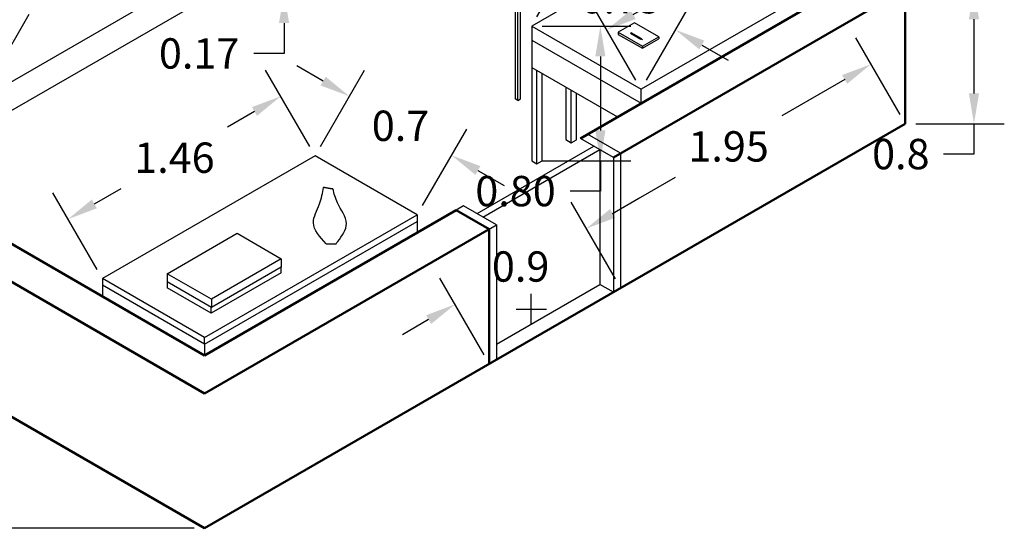
# Model space of a CAD drawing. Units: metres. Extents: x 4633 to 4644.7, y 5356.8 to 5365.2.
# Tile 2 of 3: x 4638.8 to 4644.7, y 5356.8 to 5359.9. Entities that reach past the tile are written whole.
import ezdxf

# ---------------------------------------------------------------- set-up
doc = ezdxf.new("R2010")
doc.units = ezdxf.units.M
for name, color, linetype, lineweight in [('A-ANNO-DIMS', 2, 'Continuous', 18), ('A-DOOR', 4, 'Continuous', 25), ('A-FURN', 8, 'Continuous', 25), ('A-WALL', 7, 'Continuous', 50)]:
    doc.layers.add(name, color=color, linetype=linetype, lineweight=lineweight)
doc.styles.get("Standard").update_dxf_attribs({"font": 'arial.ttf'})
doc.dimstyles.get("Standard").update_dxf_attribs({"dimtxt": 0.18, "dimasz": 0.18, "dimexe": 0.18, "dimexo": 0.0625, "dimgap": 0.09, "dimtad": 0, "dimtih": 1, "dimtoh": 1, "dimdec": 4, "dimzin": 0, "dimdsep": 46, "dimtxsty": 'Standard', "dimcen": 0.09, "dimadec": 0, "dimazin": 0, "dimtfac": 1, "dimtdec": 4, "dimtofl": 0, "dimtmove": 0, "dimatfit": 3, "dimfxl": 1, "dimtolj": 1, "dimtzin": 0, "dimarcsym": 0})

# ---------------------------------------------------------------- blocks, each defined once
blk = doc.blocks.new('*D3')
at = {"layer": 'A-ANNO-DIMS', "color": 0, "lineweight": -2, "transparency": 16777216}
for p, q in [((4639.855, 5364.6413), (4635.6927, 5364.6413)), ((4635.8727, 5364.4613), (4635.8727, 5360.9232)), ((4635.8727, 5357.0213), (4635.8727, 5360.5594)), ((4639.855, 5356.8413), (4635.6927, 5356.8413))]:
    blk.add_line(p, q, dxfattribs=at)
at = {"layer": 'A-ANNO-DIMS', "color": 0, "transparency": 16777216}
for points in [[(4635.8427, 5364.4613), (4635.9027, 5364.4613), (4635.8727, 5364.6413)], [(4635.8427, 5357.0213), (4635.9027, 5357.0213), (4635.8727, 5356.8413)]]:
    blk.add_solid(points, dxfattribs=at)
at = {"layer": 'Defpoints', "color": 0, "transparency": 16777216}
for p in [(4639.9175, 5364.6413), (4635.8727, 5356.8413), (4639.9175, 5356.8413)]:
    blk.add_point(p, dxfattribs=at)
at = {"layer": 'A-ANNO-DIMS', "color": 0, "transparency": 16777216, "insert": (4635.8727, 5360.7413), "char_height": 0.18, "attachment_point": 5}
blk.add_mtext('\\A1;7.8', dxfattribs=at)
blk = doc.blocks.new('*D6')
at = {"layer": 'A-ANNO-DIMS', "color": 0, "lineweight": -2, "transparency": 16777216}
for p, q in [((4644.1369, 5360.0413), (4644.6619, 5360.0413)), ((4644.4819, 5359.8613), (4644.4819, 5359.4213)), ((4644.1369, 5359.2413), (4644.6619, 5359.2413)), ((4644.4819, 5359.2413), (4644.4819, 5359.0613)), ((4644.4819, 5359.0613), (4644.3019, 5359.0613))]:
    blk.add_line(p, q, dxfattribs=at)
at = {"layer": 'A-ANNO-DIMS', "color": 0, "transparency": 16777216}
for points in [[(4644.4519, 5359.8613), (4644.5119, 5359.8613), (4644.4819, 5360.0413)], [(4644.4519, 5359.4213), (4644.5119, 5359.4213), (4644.4819, 5359.2413)]]:
    blk.add_solid(points, dxfattribs=at)
at = {"layer": 'Defpoints', "color": 0, "transparency": 16777216}
for p in [(4644.0744, 5360.0413), (4644.0744, 5359.2413), (4644.4819, 5359.2413)]:
    blk.add_point(p, dxfattribs=at)
at = {"layer": 'A-ANNO-DIMS', "color": 0, "transparency": 16777216, "insert": (4644.0479, 5359.0613), "char_height": 0.18, "attachment_point": 5}
blk.add_mtext('\\A1;0.8', dxfattribs=at)
blk = doc.blocks.new('*D7')
at = {"layer": 'A-ANNO-DIMS', "color": 0, "lineweight": -2, "transparency": 16777216}
for p, q in [((4642.3544, 5358.3204), (4642.0919, 5358.7751)), ((4642.3378, 5358.7092), (4642.4937, 5358.7992)), ((4641.575, 5357.8704), (4641.3125, 5358.3251)), ((4641.2466, 5358.0792), (4641.0907, 5357.9892))]:
    blk.add_line(p, q, dxfattribs=at)
at = {"layer": 'A-ANNO-DIMS', "color": 0, "transparency": 16777216}
for points in [[(4642.3228, 5358.7352), (4642.3528, 5358.6832), (4642.1819, 5358.6192)], [(4641.2316, 5358.1052), (4641.2616, 5358.0532), (4641.4025, 5358.1692)]]:
    blk.add_solid(points, dxfattribs=at)
at = {"layer": 'Defpoints', "color": 0, "transparency": 16777216}
for p in [(4642.1819, 5358.6192), (4642.3857, 5358.2663), (4641.6062, 5357.8163)]:
    blk.add_point(p, dxfattribs=at)
at = {"layer": 'A-ANNO-DIMS', "color": 0, "transparency": 16777216, "insert": (4641.7922, 5358.3942), "char_height": 0.18, "attachment_point": 5}
blk.add_mtext('\\A1;0.9', dxfattribs=at)
blk = doc.blocks.new('*D8')
at = {"layer": 'A-ANNO-DIMS', "color": 0, "lineweight": -2, "transparency": 16777216}
for p, q in [((4644.0432, 5359.2954), (4643.7807, 5359.7501)), ((4643.7148, 5359.5042), (4643.3413, 5359.2886)), ((4642.3378, 5358.7092), (4642.7112, 5358.9248)), ((4642.3544, 5358.3204), (4642.0919, 5358.7751))]:
    blk.add_line(p, q, dxfattribs=at)
at = {"layer": 'A-ANNO-DIMS', "color": 0, "transparency": 16777216}
for points in [[(4643.6998, 5359.5302), (4643.7298, 5359.4782), (4643.8707, 5359.5942)], [(4642.3228, 5358.7352), (4642.3528, 5358.6832), (4642.1819, 5358.6192)]]:
    blk.add_solid(points, dxfattribs=at)
at = {"layer": 'Defpoints', "color": 0, "transparency": 16777216}
for p in [(4643.8707, 5359.5942), (4644.0744, 5359.2413), (4642.3857, 5358.2663)]:
    blk.add_point(p, dxfattribs=at)
at = {"layer": 'A-ANNO-DIMS', "color": 0, "transparency": 16777216, "insert": (4643.0263, 5359.1067), "char_height": 0.18, "attachment_point": 5}
blk.add_mtext('\\A1;1.95', dxfattribs=at)
blk = doc.blocks.new('*D17')
at = {"layer": 'A-ANNO-DIMS', "color": 0, "lineweight": -2, "transparency": 16777216}
for p, q in [((4637.213, 5360.2454), (4637.4755, 5360.7001)), ((4637.5414, 5360.4542), (4637.771, 5360.3216)), ((4638.6308, 5359.8252), (4638.4012, 5359.9578)), ((4638.6142, 5359.4364), (4638.8767, 5359.8911))]:
    blk.add_line(p, q, dxfattribs=at)
at = {"layer": 'A-ANNO-DIMS', "color": 0, "transparency": 16777216}
for points in [[(4637.5564, 5360.4802), (4637.5264, 5360.4282), (4637.3855, 5360.5442)], [(4638.6458, 5359.8512), (4638.6158, 5359.7992), (4638.7867, 5359.7352)]]:
    blk.add_solid(points, dxfattribs=at)
at = {"layer": 'Defpoints', "color": 0, "transparency": 16777216}
for p in [(4637.1817, 5360.1913), (4638.7867, 5359.7352), (4638.583, 5359.3823)]:
    blk.add_point(p, dxfattribs=at)
at = {"layer": 'A-ANNO-DIMS', "color": 0, "transparency": 16777216, "insert": (4638.0861, 5360.1397), "char_height": 0.18, "attachment_point": 5}
blk.add_mtext('\\A1;1.618', dxfattribs=at)
blk = doc.blocks.new('*D18')
at = {"layer": 'A-ANNO-DIMS', "color": 0, "lineweight": -2, "transparency": 16777216}
for p, q in [((4639.9499, 5360.2437), (4639.6874, 5360.6983)), ((4639.6215, 5360.4524), (4639.3762, 5360.3108)), ((4638.5351, 5359.8252), (4638.7804, 5359.9668)), ((4638.5517, 5359.4364), (4638.2892, 5359.8911))]:
    blk.add_line(p, q, dxfattribs=at)
at = {"layer": 'A-ANNO-DIMS', "color": 0, "transparency": 16777216}
for points in [[(4639.6065, 5360.4784), (4639.6365, 5360.4265), (4639.7774, 5360.5424)], [(4638.5201, 5359.8512), (4638.5501, 5359.7992), (4638.3792, 5359.7352)]]:
    blk.add_solid(points, dxfattribs=at)
at = {"layer": 'Defpoints', "color": 0, "transparency": 16777216}
for p in [(4639.7774, 5360.5424), (4639.9812, 5360.1895), (4638.583, 5359.3823)]:
    blk.add_point(p, dxfattribs=at)
at = {"layer": 'A-ANNO-DIMS', "color": 0, "transparency": 16777216, "insert": (4639.0783, 5360.1388), "char_height": 0.18, "attachment_point": 5}
blk.add_mtext('\\A1;1.61', dxfattribs=at)
blk = doc.blocks.new('*D19')
at = {"layer": 'A-ANNO-DIMS', "color": 0, "lineweight": -2, "transparency": 16777216}
for p, q in [((4640.3887, 5360.3695), (4640.3887, 5360.5495)), ((4640.0437, 5360.1895), (4640.5687, 5360.1895)), ((4640.0437, 5360.0182), (4640.5687, 5360.0182)), ((4640.3887, 5359.8382), (4640.3887, 5359.6582)), ((4640.3887, 5359.6582), (4640.2087, 5359.6582))]:
    blk.add_line(p, q, dxfattribs=at)
at = {"layer": 'A-ANNO-DIMS', "color": 0, "transparency": 16777216}
for points in [[(4640.3587, 5360.3695), (4640.4187, 5360.3695), (4640.3887, 5360.1895)], [(4640.3587, 5359.8382), (4640.4187, 5359.8382), (4640.3887, 5360.0182)]]:
    blk.add_solid(points, dxfattribs=at)
at = {"layer": 'Defpoints', "color": 0, "transparency": 16777216}
for p in [(4639.9812, 5360.1895), (4639.9812, 5360.0182), (4640.3887, 5360.0182)]:
    blk.add_point(p, dxfattribs=at)
at = {"layer": 'A-ANNO-DIMS', "color": 0, "transparency": 16777216, "insert": (4639.8849, 5359.6582), "char_height": 0.18, "attachment_point": 5}
blk.add_mtext('\\A1;0.17', dxfattribs=at)
blk = doc.blocks.new('*D25')
at = {"layer": 'A-ANNO-DIMS', "color": 0, "lineweight": -2, "transparency": 16777216}
for p, q in [((4641.9058, 5360.2632), (4641.7499, 5360.3532)), ((4641.8892, 5359.8745), (4642.1517, 5360.3291)), ((4642.5387, 5359.4995), (4642.8012, 5359.9541)), ((4642.8671, 5359.7082), (4643.023, 5359.6182))]:
    blk.add_line(p, q, dxfattribs=at)
at = {"layer": 'A-ANNO-DIMS', "color": 0, "transparency": 16777216}
for points in [[(4641.9208, 5360.2892), (4641.8908, 5360.2373), (4642.0617, 5360.1732)], [(4642.8821, 5359.7342), (4642.8521, 5359.6823), (4642.7112, 5359.7982)]]:
    blk.add_solid(points, dxfattribs=at)
at = {"layer": 'Defpoints', "color": 0, "transparency": 16777216}
for p in [(4641.8579, 5359.8203), (4642.7112, 5359.7982), (4642.5075, 5359.4453)]:
    blk.add_point(p, dxfattribs=at)
at = {"layer": 'A-ANNO-DIMS', "color": 0, "transparency": 16777216, "insert": (4642.3865, 5359.9857), "char_height": 0.18, "attachment_point": 5}
blk.add_mtext('\\A1;0.75', dxfattribs=at)
blk = doc.blocks.new('*D26')
at = {"layer": 'A-ANNO-DIMS', "color": 0, "lineweight": -2, "transparency": 16777216}
for p, q in [((4643.6517, 5360.1781), (4643.3892, 5360.6328)), ((4643.3233, 5360.3869), (4643.2066, 5360.3195)), ((4642.4762, 5359.4995), (4642.2137, 5359.9541)), ((4642.4596, 5359.8882), (4642.5763, 5359.9556))]:
    blk.add_line(p, q, dxfattribs=at)
at = {"layer": 'A-ANNO-DIMS', "color": 0, "transparency": 16777216}
for points in [[(4643.3083, 5360.4129), (4643.3383, 5360.3609), (4643.4792, 5360.4769)], [(4642.4446, 5359.9142), (4642.4746, 5359.8623), (4642.3037, 5359.7982)]]:
    blk.add_solid(points, dxfattribs=at)
at = {"layer": 'Defpoints', "color": 0, "transparency": 16777216}
for p in [(4643.4792, 5360.4769), (4643.683, 5360.124), (4642.5075, 5359.4453)]:
    blk.add_point(p, dxfattribs=at)
at = {"layer": 'A-ANNO-DIMS', "color": 0, "transparency": 16777216, "insert": (4642.8915, 5360.1376), "char_height": 0.18, "attachment_point": 5}
blk.add_mtext('\\A1;1.36', dxfattribs=at)
blk = doc.blocks.new('*D27')
at = {"layer": 'A-ANNO-DIMS', "color": 0, "lineweight": -2, "transparency": 16777216}
for p, q in [((4641.9204, 5359.8203), (4642.4454, 5359.8203)), ((4642.2654, 5359.6403), (4642.2654, 5359.2016)), ((4641.9204, 5359.0216), (4642.4454, 5359.0216)), ((4642.2654, 5359.0216), (4642.2654, 5358.8416)), ((4642.2654, 5358.8416), (4642.0854, 5358.8416))]:
    blk.add_line(p, q, dxfattribs=at)
at = {"layer": 'A-ANNO-DIMS', "color": 0, "transparency": 16777216}
for points in [[(4642.2354, 5359.6403), (4642.2954, 5359.6403), (4642.2654, 5359.8203)], [(4642.2354, 5359.2016), (4642.2954, 5359.2016), (4642.2654, 5359.0216)]]:
    blk.add_solid(points, dxfattribs=at)
at = {"layer": 'Defpoints', "color": 0, "transparency": 16777216}
for p in [(4641.8579, 5359.8203), (4641.8579, 5359.0216), (4642.2654, 5359.0216)]:
    blk.add_point(p, dxfattribs=at)
at = {"layer": 'A-ANNO-DIMS', "color": 0, "transparency": 16777216, "insert": (4641.762, 5358.8416), "char_height": 0.18, "attachment_point": 5}
blk.add_mtext('\\A1;0.80', dxfattribs=at)
blk = doc.blocks.new('*D28')
at = {"layer": 'A-ANNO-DIMS', "color": 0, "lineweight": -2, "transparency": 16777216}
for p, q in [((4640.5416, 5359.1052), (4640.2791, 5359.5598)), ((4640.2132, 5359.3139), (4640.0534, 5359.2217)), ((4639.28, 5358.3768), (4639.0175, 5358.8315)), ((4639.2634, 5358.7656), (4639.4232, 5358.8579))]:
    blk.add_line(p, q, dxfattribs=at)
at = {"layer": 'A-ANNO-DIMS', "color": 0, "transparency": 16777216}
for points in [[(4640.1982, 5359.3399), (4640.2282, 5359.288), (4640.3691, 5359.4039)], [(4639.2484, 5358.7916), (4639.2784, 5358.7396), (4639.1075, 5358.6756)]]:
    blk.add_solid(points, dxfattribs=at)
at = {"layer": 'Defpoints', "color": 0, "transparency": 16777216}
for p in [(4640.3691, 5359.4039), (4640.5728, 5359.051), (4639.3113, 5358.3227)]:
    blk.add_point(p, dxfattribs=at)
at = {"layer": 'A-ANNO-DIMS', "color": 0, "transparency": 16777216, "insert": (4639.7383, 5359.0398), "char_height": 0.18, "attachment_point": 5}
blk.add_mtext('\\A1;1.46', dxfattribs=at)
blk = doc.blocks.new('*D29')
at = {"layer": 'A-ANNO-DIMS', "color": 0, "lineweight": -2, "transparency": 16777216}
for p, q in [((4640.6207, 5359.4939), (4640.4648, 5359.5839)), ((4640.6041, 5359.1052), (4640.8666, 5359.5598)), ((4641.2103, 5358.7552), (4641.4728, 5359.2098)), ((4641.5387, 5358.9639), (4641.6946, 5358.8739))]:
    blk.add_line(p, q, dxfattribs=at)
at = {"layer": 'A-ANNO-DIMS', "color": 0, "transparency": 16777216}
for points in [[(4640.6357, 5359.5199), (4640.6057, 5359.468), (4640.7766, 5359.4039)], [(4641.5537, 5358.9899), (4641.5237, 5358.938), (4641.3828, 5359.0539)]]:
    blk.add_solid(points, dxfattribs=at)
at = {"layer": 'Defpoints', "color": 0, "transparency": 16777216}
for p in [(4641.3828, 5359.0539), (4640.5728, 5359.051), (4641.1791, 5358.701)]:
    blk.add_point(p, dxfattribs=at)
at = {"layer": 'A-ANNO-DIMS', "color": 0, "transparency": 16777216, "insert": (4641.0797, 5359.2289), "char_height": 0.18, "attachment_point": 5}
blk.add_mtext('\\A1;0.7', dxfattribs=at)
blk = doc.blocks.new('*D30')
at = {"layer": 'A-ANNO-DIMS', "color": 0, "lineweight": -2, "transparency": 16777216}
for p, q in [((4633.8236, 5361.0144), (4634.0036, 5361.0144)), ((4634.0036, 5361.0144), (4636.779, 5359.9989)), ((4641.8554, 5358.0514), (4641.8554, 5358.2314)), ((4641.7654, 5358.1414), (4641.9454, 5358.1414))]:
    blk.add_line(p, q, dxfattribs=at)
at = {"layer": 'A-ANNO-DIMS', "color": 0, "transparency": 16777216}
blk.add_solid([(4636.7893, 5360.027), (4636.7686, 5359.9707), (4636.948, 5359.937)], dxfattribs=at)
at = {"layer": 'Defpoints', "color": 0, "transparency": 16777216}
for p in [(4636.948, 5359.937), (4641.8554, 5358.1414)]:
    blk.add_point(p, dxfattribs=at)
at = {"layer": 'A-ANNO-DIMS', "color": 0, "transparency": 16777216, "insert": (4633.3438, 5361.0144), "char_height": 0.18, "attachment_point": 5}
blk.add_mtext('\\A1;R5.226', dxfattribs=at)

msp = doc.modelspace()

# ---------------------------------------------------------------- linework, layer by layer
at = {"layer": 'A-DOOR'}
for p, q in [((4642.3857, 5359.0663), (4642.1899, 5359.1793)), ((4642.3424, 5359.0413), (4642.1466, 5359.1543)), ((4641.5344, 5358.7078), (4642.2272, 5359.1078)), ((4641.569, 5358.6878), (4642.2618, 5359.0878)), ((4642.2618, 5359.0878), (4642.2618, 5358.2878)), ((4642.3857, 5359.0663), (4642.3857, 5358.2663)), ((4642.3424, 5359.0413), (4642.3424, 5358.2413)), ((4641.4538, 5358.7543), (4641.4105, 5358.7293)), ((4641.6495, 5358.6413), (4641.4538, 5358.7543)), ((4641.6062, 5358.6163), (4641.6495, 5358.6413)), ((4641.6495, 5358.6413), (4641.6495, 5357.8413)), ((4641.6495, 5357.9343), (4642.2618, 5358.2878)), ((4642.3424, 5358.2413), (4642.2618, 5358.2878))]:
    msp.add_line(p, q, dxfattribs=at)
at = {"layer": 'A-FURN'}
for p, q in [((4643.0334, 5360.499), (4641.8579, 5359.8203)), ((4638.583, 5359.3823), (4639.9812, 5360.1895)), ((4643.683, 5360.124), (4642.5075, 5359.4453)), ((4638.583, 5359.2109), (4639.9812, 5360.0182)), ((4641.7594, 5359.9907), (4641.7594, 5359.388)), ((4641.7751, 5359.3789), (4641.7751, 5359.9822)), ((4641.7922, 5359.3888), (4641.7922, 5359.9729)), ((4641.8579, 5359.8203), (4642.5075, 5359.4453)), ((4641.8579, 5359.8203), (4641.8579, 5359.7376)), ((4642.4684, 5359.8395), (4642.3718, 5359.7837)), ((4642.6114, 5359.757), (4642.4684, 5359.8395)), ((4642.3718, 5359.7837), (4642.5148, 5359.7012)), ((4642.3718, 5359.7837), (4642.3718, 5359.7715)), ((4642.3718, 5359.7715), (4642.5148, 5359.689)), ((4642.4475, 5359.7805), (4642.4444, 5359.7787)), ((4642.4444, 5359.7787), (4642.5054, 5359.7435)), ((4642.5077, 5359.7458), (4642.4475, 5359.7805)), ((4642.5148, 5359.7012), (4642.6114, 5359.757)), ((4642.6114, 5359.757), (4642.6114, 5359.7448)), ((4641.8579, 5359.7376), (4642.5075, 5359.3626)), ((4641.8579, 5359.7376), (4641.8579, 5359.5754)), ((4642.5054, 5359.7435), (4642.5077, 5359.7458)), ((4642.5161, 5359.7391), (4642.5054, 5359.7435)), ((4642.5161, 5359.7391), (4642.5077, 5359.7458)), ((4642.5148, 5359.689), (4642.6114, 5359.7448)), ((4642.5148, 5359.7012), (4642.5148, 5359.689)), ((4641.8579, 5359.5754), (4642.367, 5359.2815)), ((4641.8579, 5359.5754), (4641.8579, 5359.0216)), ((4641.8894, 5359.0034), (4641.8894, 5359.5572)), ((4641.9199, 5359.021), (4641.9199, 5359.5396)), ((4642.0613, 5359.458), (4642.0613, 5359.147)), ((4642.0928, 5359.1288), (4642.0928, 5359.4398)), ((4642.1233, 5359.1464), (4642.1233, 5359.4222)), ((4642.5075, 5359.3626), (4642.5075, 5359.4453)), ((4641.7751, 5359.3789), (4641.7594, 5359.388)), ((4641.7751, 5359.3789), (4641.7922, 5359.3888)), ((4642.0613, 5359.147), (4642.0928, 5359.1288)), ((4642.0928, 5359.1288), (4642.1233, 5359.1464)), ((4640.5728, 5359.051), (4639.3113, 5358.3227)), ((4641.1791, 5358.701), (4640.5728, 5359.051)), ((4641.8579, 5359.0216), (4641.8894, 5359.0034)), ((4641.8894, 5359.0034), (4641.9199, 5359.021)), ((4639.9175, 5357.9727), (4641.1791, 5358.701)), ((4639.9175, 5357.9329), (4641.1791, 5358.6613)), ((4641.1791, 5358.701), (4641.1791, 5358.6613)), ((4641.1791, 5358.6613), (4641.1791, 5358.5957)), ((4639.6952, 5358.3517), (4640.11, 5358.5911)), ((4640.11, 5358.5911), (4640.3725, 5358.4396)), ((4640.6395, 5358.5294), (4640.6982, 5358.5297)), ((4640.3725, 5358.4396), (4639.9577, 5358.2001)), ((4640.3725, 5358.4396), (4640.3725, 5358.3906)), ((4640.3716, 5358.356), (4639.9568, 5358.1165)), ((4640.3725, 5358.3906), (4639.9577, 5358.1511)), ((4640.3716, 5358.356), (4640.3716, 5358.3901)), ((4639.9175, 5357.9727), (4639.3113, 5358.3227)), ((4639.3113, 5358.3227), (4639.3113, 5358.2829)), ((4639.6952, 5358.3027), (4639.6943, 5358.2681)), ((4639.9577, 5358.2001), (4639.6952, 5358.3517)), ((4639.6952, 5358.3517), (4639.6952, 5358.3027)), ((4639.9577, 5358.1511), (4639.6952, 5358.3027)), ((4639.9175, 5357.9329), (4639.3113, 5358.2829)), ((4639.3113, 5358.2829), (4639.3113, 5358.2173)), ((4639.9568, 5358.1165), (4639.6943, 5358.2681)), ((4639.9577, 5358.2001), (4639.9577, 5358.1511)), ((4639.9568, 5358.1165), (4639.9568, 5358.1516)), ((4639.9175, 5357.9329), (4639.9175, 5357.9727)), ((4639.9175, 5357.9329), (4639.9175, 5357.8673))]:
    msp.add_line(p, q, dxfattribs=at)
msp.add_ellipse((4640.6508, 5358.8594), major_axis=(-0.0281, 0.0042), ratio=0.077616, dxfattribs=at)
for points, knots in [([(4640.6395, 5358.5294), (4640.6017, 5358.5695), (4640.5332, 5358.6419), (4640.6054, 5358.7599), (4640.6172, 5358.8309), (4640.6227, 5358.8636)], [0, 0, 0, 0, 0.1459343, 0.2637327, 0.3644883, 0.3644883, 0.3644883, 0.3644883]), ([(4640.6982, 5358.5297), (4640.7012, 5358.5337), (4640.7041, 5358.5377), (4640.7071, 5358.5417), (4640.7071, 5358.5417), (4640.7071, 5358.5417), (4640.7071, 5358.5417), (4640.7333, 5358.5774), (4640.789, 5358.6532), (4640.7032, 5358.7563), (4640.6858, 5358.8272), (4640.6789, 5358.8552)], [-0.0134388, -0.0134388, -0.0134388, -0.0134388, 0, 0, 0, 0, 0, 0, 0.1192983, 0.253158, 0.3409363, 0.3409363, 0.3409363, 0.3409363])]:
    msp.add_open_spline(points, degree=3, knots=knots, dxfattribs=at)
at = {"layer": 'A-WALL'}
for p, q in [((4644.0744, 5362.2413), (4644.0744, 5359.2413)), ((4642.1466, 5359.1543), (4643.683, 5360.0413)), ((4642.3424, 5359.0413), (4644.0744, 5360.0413)), ((4636.6716, 5359.7413), (4639.9175, 5357.8673)), ((4639.9175, 5357.6413), (4636.4759, 5359.6283)), ((4639.9175, 5356.8413), (4644.0744, 5359.2413)), ((4636.2802, 5358.9413), (4639.9175, 5356.8413)), ((4639.9175, 5357.8673), (4641.4105, 5358.7293)), ((4641.6062, 5358.6163), (4641.4105, 5358.7293)), ((4639.9175, 5357.6413), (4641.6062, 5358.6163)), ((4641.6062, 5358.6163), (4641.6062, 5357.8163))]:
    msp.add_line(p, q, dxfattribs=at)

# ---------------------------------------------------------------- dimensions: what is measured, and where the dimension line sits
at = {"layer": 'A-ANNO-DIMS'}
for base, p1, p2, angle, override, picture, middle in [((4635.8727, 5356.8413), (4639.9175, 5364.6413), (4639.9175, 5356.8413), 90, {"dimdec": 1, "dimlfac": 1, "dimrnd": 0, "dimzin": 0, "dimdsep": 46, "dimlunit": 2}, '*D3', (4635.8727, 5360.7413)), ((4638.7867, 5359.7352), (4637.1817, 5360.1913), (4638.583, 5359.3823), 330, {"dimdec": 3, "dimlfac": 1, "dimrnd": 0, "dimzin": 0, "dimdsep": 46, "dimlunit": 2}, '*D17', (4638.0861, 5360.1397)), ((4639.7774, 5360.5424), (4638.583, 5359.3823), (4639.9812, 5360.1895), 30, {"dimdec": 2, "dimlfac": 1, "dimrnd": 0, "dimzin": 0, "dimdsep": 46, "dimlunit": 2}, '*D18', (4639.0783, 5360.1388)), ((4643.4792, 5360.4769), (4642.5075, 5359.4453), (4643.683, 5360.124), 30, {"dimdec": 2, "dimlfac": 1, "dimrnd": 0, "dimzin": 0, "dimdsep": 46, "dimlunit": 2}, '*D26', (4642.8915, 5360.1376)), ((4640.3887, 5360.0182), (4639.9812, 5360.1895), (4639.9812, 5360.0182), 270, {"dimdec": 2, "dimlfac": 1, "dimrnd": 0, "dimzin": 0, "dimdsep": 46, "dimlunit": 2}, '*D19', (4639.8849, 5359.6582)), ((4642.7112, 5359.7982), (4641.8579, 5359.8203), (4642.5075, 5359.4453), 330, {"dimdec": 2, "dimlfac": 1, "dimrnd": 0, "dimzin": 0, "dimdsep": 46, "dimlunit": 2}, '*D25', (4642.3865, 5359.9857)), ((4644.4819, 5359.2413), (4644.0744, 5360.0413), (4644.0744, 5359.2413), 270, {"dimdec": 1, "dimlfac": 1, "dimrnd": 0, "dimzin": 0, "dimdsep": 46, "dimlunit": 2}, '*D6', (4644.0479, 5359.0613)), ((4642.2654, 5359.0216), (4641.8579, 5359.8203), (4641.8579, 5359.0216), 270, {"dimdec": 2, "dimlfac": 1, "dimrnd": 0, "dimzin": 0, "dimdsep": 46, "dimlunit": 2}, '*D27', (4641.762, 5358.8416)), ((4643.8707, 5359.5942), (4642.3857, 5358.2663), (4644.0744, 5359.2413), 30, {"dimdec": 2, "dimlfac": 1, "dimrnd": 0, "dimzin": 0, "dimdsep": 46, "dimlunit": 2}, '*D8', (4643.0263, 5359.1067)), ((4641.3828, 5359.0539), (4640.5728, 5359.051), (4641.1791, 5358.701), 330, {"dimdec": 1, "dimlfac": 1, "dimrnd": 0, "dimzin": 0, "dimdsep": 46, "dimlunit": 2}, '*D29', (4641.0797, 5359.2289)), ((4640.3691, 5359.4039), (4639.3113, 5358.3227), (4640.5728, 5359.051), 30, {"dimdec": 2, "dimlfac": 1, "dimrnd": 0, "dimzin": 0, "dimdsep": 46, "dimlunit": 2}, '*D28', (4639.7383, 5359.0398)), ((4642.1819, 5358.6192), (4641.6062, 5357.8163), (4642.3857, 5358.2663), 30, {"dimdec": 1, "dimlfac": 1, "dimrnd": 0, "dimzin": 0, "dimdsep": 46, "dimlunit": 2}, '*D7', (4641.7922, 5358.3942))]:
    dim = msp.add_linear_dim(base=base, p1=p1, p2=p2, angle=angle, dimstyle='Standard', override=override, dxfattribs=at)
    dim.commit()
    dim.dimension.update_dxf_attribs({"geometry": picture, "text_midpoint": middle})
dim = msp.add_radius_dim(center=(4641.8554, 5358.1414), mpoint=(4636.948, 5359.937), dimstyle='Standard', override={"dimdec": 3, "dimlfac": 1, "dimrnd": 0, "dimzin": 0, "dimdsep": 46, "dimlunit": 2}, dxfattribs=at)
dim.commit()
dim.dimension.update_dxf_attribs({"geometry": '*D30', "text_midpoint": (4633.3438, 5361.0144), "dimtype": 164})

doc.saveas('drawing.dxf')
